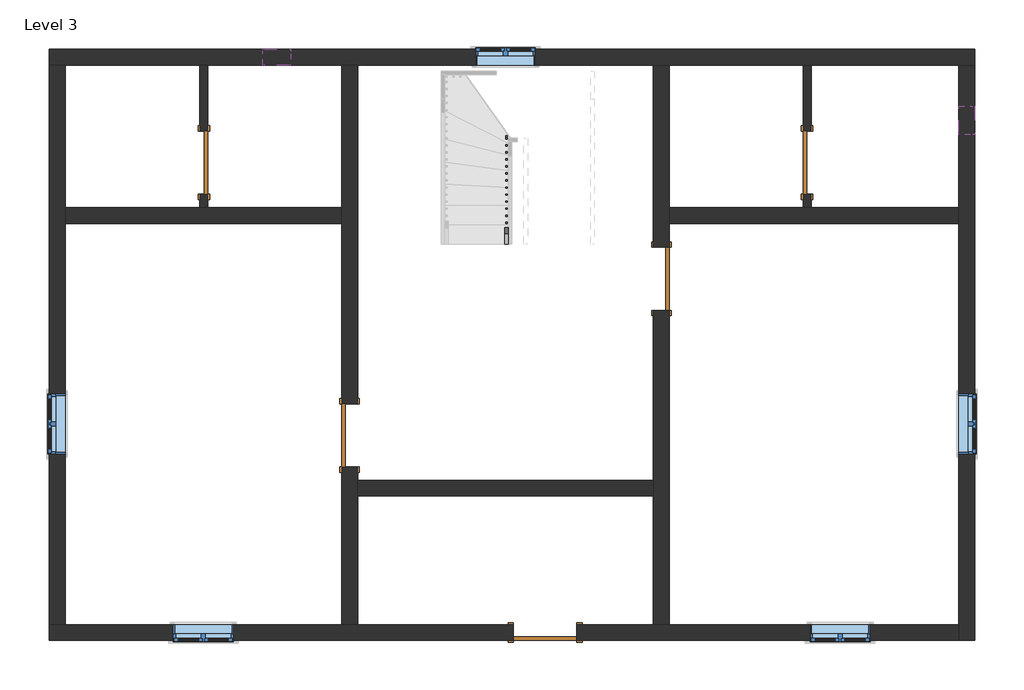
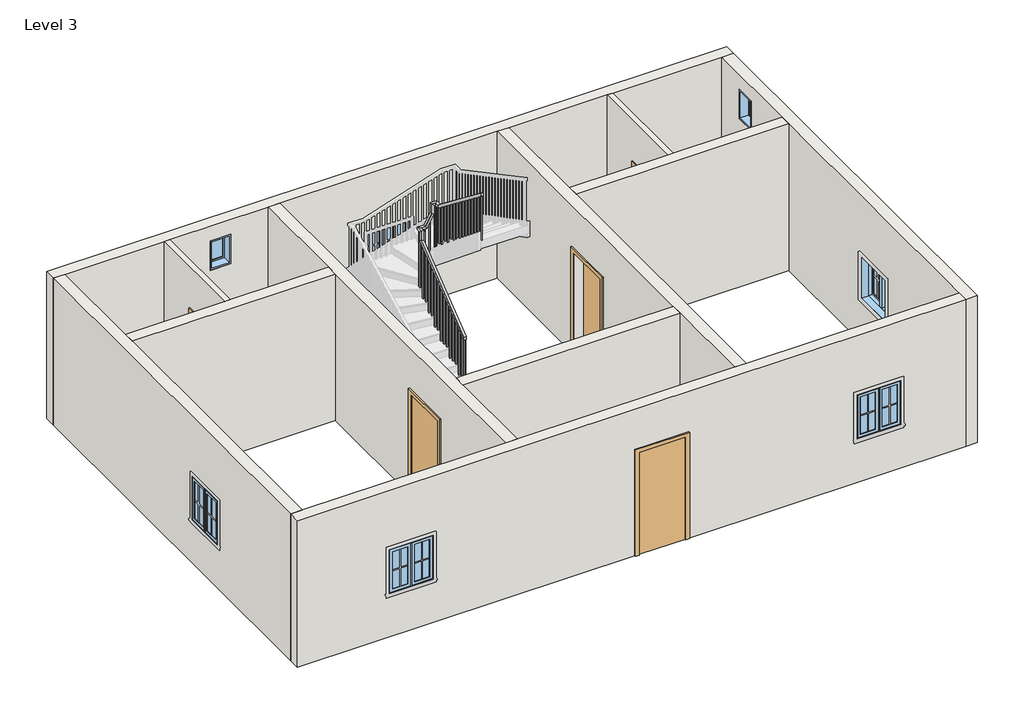
# One storey, part 1 of 2: 11 walls, 7 windows, 5 doors, 1 railing.
"""IFC4 building model written with IfcOpenShell, lengths in millimetres."""

from ifc_helpers import new_model, si_unit, frame, origin, place, context, project, spatial, polyline, outline, extrude, faceted_brep, transform, mapped, element, save
from components import door_e5f9f3c4, door_a90ba1ad, door_305aa2a5, door_0ca8825f, window_aa618e30, window_339605e1

model = new_model("IFC4")

# Units and contexts
model_context = context("Model", 3, world=origin())
ifc_project = project(units=[si_unit("LENGTHUNIT", "METRE", prefix="MILLI")], contexts=[model_context])

# Site, building, storey
site = spatial("IfcSite", under=ifc_project)
building = spatial("IfcBuilding", under=site)
storey = spatial("IfcBuildingStorey", under=building, Name="Level 3", Elevation=3200.4)

# Doors
placement = place(None, origin())
door_shape = door_e5f9f3c4(model_context)
element("IfcDoor", 1, ObjectType="Single-Flush : 36\" x 84\"", at=placement, inside=storey, context=model_context, shape_type="MappedRepresentation", body=[
    mapped(door_shape, transform((-5102.9390964, 4820.103532, 3200.4), x_axis=(0.0, -1.0, 0.0), y_axis=(1.0, 0.0, 0.0), z_axis=(0.0, 0.0, 1.0))),
])
door_2_shape = door_a90ba1ad(model_context)
element("IfcDoor", 2, ObjectType="Single-Flush : 36\" x 84\"", at=placement, inside=storey, context=model_context, shape_type="MappedRepresentation", body=[
    mapped(door_2_shape, transform((-3001.0890964, 883.103532, 3200.4), x_axis=(0.0, -1.0, 0.0), y_axis=(1.0, 0.0, 0.0), z_axis=(0.0, 0.0, 1.0))),
])
element("IfcDoor", 3, ObjectType="Single-Flush : 36\" x 84\"", at=placement, inside=storey, context=model_context, shape_type="MappedRepresentation", body=[
    mapped(door_2_shape, transform((1494.7109036, 3143.703532, 3200.4), x_axis=(0.0, 1.0, 0.0), y_axis=(-1.0, 0.0, 0.0), z_axis=(0.0, 0.0, 1.0))),
])
door_3_shape = door_305aa2a5(model_context)
element("IfcDoor", 4, ObjectType="Single-Flush : 36\" x 84\"", at=placement, inside=storey, context=model_context, shape_type="MappedRepresentation", body=[
    mapped(door_3_shape, transform((3596.5609036, 4820.103532, 3200.4), x_axis=(0.0, -1.0, 0.0), y_axis=(1.0, 0.0, 0.0), z_axis=(0.0, 0.0, 1.0))),
])
door_4_shape = door_0ca8825f(model_context)
element("IfcDoor", 5, ObjectType="Single-Flush : 36\" x 84\"", at=placement, inside=storey, context=model_context, shape_type="MappedRepresentation", body=[
    mapped(door_4_shape, transform((-181.6890964, -1961.696468, 3200.4), x_axis=(-1.0, 0.0, 0.0), y_axis=(0.0, -1.0, 0.0), z_axis=(0.0, 0.0, 1.0))),
])

# Railing
element("IfcRailing", 6, ObjectType="Handrail - Rectangular", at=placement, inside=storey, context=model_context, shape_type="SolidModel", body=[
    faceted_brep([(-765.8890964, 3647.9718401, 4284.1333333), (-765.8890964, 3647.9718401, 4219.8000346), (-715.0890964, 3647.9718401, 4219.8000346), (-715.0890964, 3647.9718401, 4284.1333333), (-765.8890964, 5099.503532, 5412.0191036), (-765.8890964, 5150.303532, 5387.1590024), (-715.0890964, 5150.303532, 5387.1590024), (-715.0890964, 5099.503532, 5412.0191036), (-765.8890964, 5099.503532, 5615.0281882), (-765.8890964, 5150.303532, 5564.2281882), (-715.0890964, 5150.303532, 5564.2281882), (-715.0890964, 5099.503532, 5615.0281882), (-765.8890964, 5226.503532, 5615.0281882), (-765.8890964, 5226.503532, 5564.2281882), (-715.0890964, 5175.703532, 5564.2281882), (-715.0890964, 5175.703532, 5615.0281882), (-638.8890964, 5226.503532, 5615.0281882), (-609.7677625, 5226.503532, 5564.2281882), (-609.7677625, 5175.703532, 5564.2281882), (-638.8890964, 5175.703532, 5615.0281882), (-511.8890964, 5226.503532, 5831.9051451), (-461.0890964, 5226.503532, 5818.1256424), (-461.0890964, 5175.703532, 5818.1256424), (-511.8890964, 5175.703532, 5831.9051451), (-511.8890964, 5226.503532, 6034.9142297), (-461.0890964, 5226.503532, 5984.1142297), (-461.0890964, 5175.703532, 5984.1142297), (-511.8890964, 5175.703532, 6034.9142297), (-384.8890964, 5226.503532, 6034.9142297), (-384.8890964, 5226.503532, 5984.1142297), (-435.6890964, 5175.703532, 5984.1142297), (-435.6890964, 5175.703532, 6034.9142297), (-384.8890964, 5099.503532, 6034.9142297), (-384.8890964, 5082.086864, 5984.1142297), (-435.6890964, 5082.086864, 5984.1142297), (-435.6890964, 5099.503532, 6034.9142297), (-384.8890964, 3647.9718401, 7162.8), (-435.6890964, 3647.9718401, 7162.8), (-435.6890964, 3647.9718401, 7098.4667013), (-384.8890964, 3647.9718401, 7098.4667013)], [[[0, 1, 2, 3]], [[1, 0, 4, 5]], [[2, 1, 5, 6]], [[3, 2, 6, 7]], [[0, 3, 7, 4]], [[5, 4, 8, 9]], [[6, 5, 9, 10]], [[7, 6, 10, 11]], [[4, 7, 11, 8]], [[9, 8, 12, 13]], [[10, 9, 13, 14]], [[11, 10, 14, 15]], [[8, 11, 15, 12]], [[13, 12, 16, 17]], [[14, 13, 17, 18]], [[15, 14, 18, 19]], [[12, 15, 19, 16]], [[17, 16, 20, 21]], [[18, 17, 21, 22]], [[19, 18, 22, 23]], [[16, 19, 23, 20]], [[21, 20, 24, 25]], [[22, 21, 25, 26]], [[23, 22, 26, 27]], [[20, 23, 27, 24]], [[25, 24, 28, 29]], [[26, 25, 29, 30]], [[27, 26, 30, 31]], [[24, 27, 31, 28]], [[29, 28, 32, 33]], [[30, 29, 33, 34]], [[31, 30, 34, 35]], [[28, 31, 35, 32]], [[36, 37, 38, 39]], [[33, 32, 36, 39]], [[34, 33, 39, 38]], [[35, 34, 38, 37]], [[32, 35, 37, 36]]]),
    extrude(outline(polyline([(3667.578532, 7083.2316852), (3686.628532, 7068.4292361), (3686.628532, 6079.0666667), (3667.578532, 6079.0666667), (3667.578532, 7083.2316852)])), frame((-419.8140964, 0.0, 0.0), z_axis=(1.0, 0.0, 0.0), x_axis=(0.0, 1.0, 0.0)), (0.0, 0.0, 1.0), 19.05),
    extrude(outline(polyline([(3769.178532, 7004.2852902), (3788.228532, 6989.4828411), (3788.228532, 6079.0666667), (3769.178532, 6079.0666667), (3769.178532, 7004.2852902)])), frame((-419.8140964, 0.0, 0.0), z_axis=(1.0, 0.0, 0.0), x_axis=(0.0, 1.0, 0.0)), (0.0, 0.0, 1.0), 19.05),
    extrude(outline(polyline([(3870.778532, 6925.3388952), (3889.828532, 6910.5364462), (3889.828532, 6079.0666667), (3870.778532, 6079.0666667), (3870.778532, 6925.3388952)])), frame((-419.8140964, 0.0, 0.0), z_axis=(1.0, 0.0, 0.0), x_axis=(0.0, 1.0, 0.0)), (0.0, 0.0, 1.0), 19.05),
    extrude(outline(polyline([(3972.378532, 6846.3925003), (3991.428532, 6831.5900512), (3991.428532, 5909.7333333), (3972.378532, 5909.7333333), (3972.378532, 6846.3925003)])), frame((-419.8140964, 0.0, 0.0), z_axis=(1.0, 0.0, 0.0), x_axis=(0.0, 1.0, 0.0)), (0.0, 0.0, 1.0), 19.05),
    extrude(outline(polyline([(4073.978532, 6767.4461053), (4093.028532, 6752.6436562), (4093.028532, 5909.7333333), (4073.978532, 5909.7333333), (4073.978532, 6767.4461053)])), frame((-419.8140964, 0.0, 0.0), z_axis=(1.0, 0.0, 0.0), x_axis=(0.0, 1.0, 0.0)), (0.0, 0.0, 1.0), 19.05),
    extrude(outline(polyline([(4175.578532, 6688.4997103), (4194.628532, 6673.6972613), (4194.628532, 5909.7333333), (4175.578532, 5909.7333333), (4175.578532, 6688.4997103)])), frame((-419.8140964, 0.0, 0.0), z_axis=(1.0, 0.0, 0.0), x_axis=(0.0, 1.0, 0.0)), (0.0, 0.0, 1.0), 19.05),
    extrude(outline(polyline([(4277.178532, 6609.5533154), (4296.228532, 6594.7508663), (4296.228532, 5740.4), (4277.178532, 5740.4), (4277.178532, 6609.5533154)])), frame((-419.8140964, 0.0, 0.0), z_axis=(1.0, 0.0, 0.0), x_axis=(0.0, 1.0, 0.0)), (0.0, 0.0, 1.0), 19.05),
    extrude(outline(polyline([(4378.778532, 6530.6069204), (4397.828532, 6515.8044713), (4397.828532, 5740.4), (4378.778532, 5740.4), (4378.778532, 6530.6069204)])), frame((-419.8140964, 0.0, 0.0), z_axis=(1.0, 0.0, 0.0), x_axis=(0.0, 1.0, 0.0)), (0.0, 0.0, 1.0), 19.05),
    extrude(outline(polyline([(4480.378532, 6451.6605254), (4499.428532, 6436.8580764), (4499.428532, 5571.0666667), (4480.378532, 5571.0666667), (4480.378532, 6451.6605254)])), frame((-419.8140964, 0.0, 0.0), z_axis=(1.0, 0.0, 0.0), x_axis=(0.0, 1.0, 0.0)), (0.0, 0.0, 1.0), 19.05),
    extrude(outline(polyline([(4581.978532, 6372.7141304), (4601.028532, 6357.9116814), (4601.028532, 5571.0666667), (4581.978532, 5571.0666667), (4581.978532, 6372.7141304)])), frame((-419.8140964, 0.0, 0.0), z_axis=(1.0, 0.0, 0.0), x_axis=(0.0, 1.0, 0.0)), (0.0, 0.0, 1.0), 19.05),
    extrude(outline(polyline([(4683.578532, 6293.7677355), (4702.628532, 6278.9652864), (4702.628532, 5571.0666667), (4683.578532, 5571.0666667), (4683.578532, 6293.7677355)])), frame((-419.8140964, 0.0, 0.0), z_axis=(1.0, 0.0, 0.0), x_axis=(0.0, 1.0, 0.0)), (0.0, 0.0, 1.0), 19.05),
    extrude(outline(polyline([(4785.178532, 6214.8213405), (4804.228532, 6200.0188914), (4804.228532, 5401.7333333), (4785.178532, 5401.7333333), (4785.178532, 6214.8213405)])), frame((-419.8140964, 0.0, 0.0), z_axis=(1.0, 0.0, 0.0), x_axis=(0.0, 1.0, 0.0)), (0.0, 0.0, 1.0), 19.05),
    extrude(outline(polyline([(4886.778532, 6135.8749455), (4905.828532, 6121.0724965), (4905.828532, 5401.7333333), (4886.778532, 5401.7333333), (4886.778532, 6135.8749455)])), frame((-419.8140964, 0.0, 0.0), z_axis=(1.0, 0.0, 0.0), x_axis=(0.0, 1.0, 0.0)), (0.0, 0.0, 1.0), 19.05),
    extrude(outline(polyline([(4988.378532, 6056.9285506), (5007.428532, 6042.1261015), (5007.428532, 5232.4), (4988.378532, 5232.4), (4988.378532, 6056.9285506)])), frame((-419.8140964, 0.0, 0.0), z_axis=(1.0, 0.0, 0.0), x_axis=(0.0, 1.0, 0.0)), (0.0, 0.0, 1.0), 19.05),
    extrude(outline(polyline([(5089.978532, 5977.9821556), (5109.028532, 5963.1797065), (5109.028532, 5232.4), (5089.978532, 5232.4), (5089.978532, 5977.9821556)])), frame((-419.8140964, 0.0, 0.0), z_axis=(1.0, 0.0, 0.0), x_axis=(0.0, 1.0, 0.0)), (0.0, 0.0, 1.0), 19.05),
    extrude(outline(polyline([(-445.2140964, 5191.578532), (-445.2140964, 5210.628532), (-426.1640964, 5210.628532), (-426.1640964, 5191.578532), (-445.2140964, 5191.578532)])), frame((0.0, 0.0, 4893.7333333), z_axis=(0.0, 0.0, 1.0), x_axis=(1.0, 0.0, 0.0)), (0.0, 0.0, 1.0), 1090.3808964),
    extrude(outline(polyline([(5704.26524, -527.7640964), (5671.7336964, -546.8140964), (4724.4, -546.8140964), (4724.4, -527.7640964), (5704.26524, -527.7640964)])), frame((0.0, 5191.578532, 0.0), z_axis=(0.0, 1.0, 0.0), x_axis=(0.0, 0.0, 1.0)), (0.0, 0.0, 1.0), 19.05),
    extrude(outline(polyline([(5530.7636744, -629.3640964), (5498.2321309, -648.4140964), (4555.0666667, -648.4140964), (4555.0666667, -629.3640964), (5530.7636744, -629.3640964)])), frame((0.0, 5191.578532, 0.0), z_axis=(0.0, 1.0, 0.0), x_axis=(0.0, 0.0, 1.0)), (0.0, 0.0, 1.0), 19.05),
    extrude(outline(polyline([(-730.9640964, 5162.4468401), (-750.0140964, 5162.4468401), (-750.0140964, 5181.4968401), (-730.9640964, 5181.4968401), (-730.9640964, 5162.4468401)])), frame((0.0, 0.0, 4385.7333333), z_axis=(0.0, 0.0, 1.0), x_axis=(1.0, 0.0, 0.0)), (0.0, 0.0, 1.0), 1178.4948549),
    extrude(outline(polyline([(5060.8468401, 5317.6483397), (5079.8968401, 5332.4507888), (5079.8968401, 4216.4), (5060.8468401, 4216.4), (5060.8468401, 5317.6483397)])), frame((-750.0140964, 0.0, 0.0), z_axis=(1.0, 0.0, 0.0), x_axis=(0.0, 1.0, 0.0)), (0.0, 0.0, 1.0), 19.05),
    extrude(outline(polyline([(4959.2468401, 5238.7019447), (4978.2968401, 5253.5043938), (4978.2968401, 4216.4), (4959.2468401, 4216.4), (4959.2468401, 5238.7019447)])), frame((-750.0140964, 0.0, 0.0), z_axis=(1.0, 0.0, 0.0), x_axis=(0.0, 1.0, 0.0)), (0.0, 0.0, 1.0), 19.05),
    extrude(outline(polyline([(4857.6468401, 5159.7555498), (4876.6968401, 5174.5579988), (4876.6968401, 4047.0666667), (4857.6468401, 4047.0666667), (4857.6468401, 5159.7555498)])), frame((-750.0140964, 0.0, 0.0), z_axis=(1.0, 0.0, 0.0), x_axis=(0.0, 1.0, 0.0)), (0.0, 0.0, 1.0), 19.05),
    extrude(outline(polyline([(4756.0468401, 5080.8091548), (4775.0968401, 5095.6116039), (4775.0968401, 4047.0666667), (4756.0468401, 4047.0666667), (4756.0468401, 5080.8091548)])), frame((-750.0140964, 0.0, 0.0), z_axis=(1.0, 0.0, 0.0), x_axis=(0.0, 1.0, 0.0)), (0.0, 0.0, 1.0), 19.05),
    extrude(outline(polyline([(4654.4468401, 5001.8627598), (4673.4968401, 5016.6652089), (4673.4968401, 3877.7333333), (4654.4468401, 3877.7333333), (4654.4468401, 5001.8627598)])), frame((-750.0140964, 0.0, 0.0), z_axis=(1.0, 0.0, 0.0), x_axis=(0.0, 1.0, 0.0)), (0.0, 0.0, 1.0), 19.05),
    extrude(outline(polyline([(4552.8468401, 4922.9163649), (4571.8968401, 4937.7188139), (4571.8968401, 3877.7333333), (4552.8468401, 3877.7333333), (4552.8468401, 4922.9163649)])), frame((-750.0140964, 0.0, 0.0), z_axis=(1.0, 0.0, 0.0), x_axis=(0.0, 1.0, 0.0)), (0.0, 0.0, 1.0), 19.05),
    extrude(outline(polyline([(4451.2468401, 4843.9699699), (4470.2968401, 4858.7724189), (4470.2968401, 3708.4), (4451.2468401, 3708.4), (4451.2468401, 4843.9699699)])), frame((-750.0140964, 0.0, 0.0), z_axis=(1.0, 0.0, 0.0), x_axis=(0.0, 1.0, 0.0)), (0.0, 0.0, 1.0), 19.05),
    extrude(outline(polyline([(4349.6468401, 4765.0235749), (4368.6968401, 4779.826024), (4368.6968401, 3708.4), (4349.6468401, 3708.4), (4349.6468401, 4765.0235749)])), frame((-750.0140964, 0.0, 0.0), z_axis=(1.0, 0.0, 0.0), x_axis=(0.0, 1.0, 0.0)), (0.0, 0.0, 1.0), 19.05),
    extrude(outline(polyline([(4248.0468401, 4686.0771799), (4267.0968401, 4700.879629), (4267.0968401, 3708.4), (4248.0468401, 3708.4), (4248.0468401, 4686.0771799)])), frame((-750.0140964, 0.0, 0.0), z_axis=(1.0, 0.0, 0.0), x_axis=(0.0, 1.0, 0.0)), (0.0, 0.0, 1.0), 19.05),
    extrude(outline(polyline([(4146.4468401, 4607.130785), (4165.4968401, 4621.933234), (4165.4968401, 3539.0666667), (4146.4468401, 3539.0666667), (4146.4468401, 4607.130785)])), frame((-750.0140964, 0.0, 0.0), z_axis=(1.0, 0.0, 0.0), x_axis=(0.0, 1.0, 0.0)), (0.0, 0.0, 1.0), 19.05),
    extrude(outline(polyline([(4044.8468401, 4528.18439), (4063.8968401, 4542.9868391), (4063.8968401, 3539.0666667), (4044.8468401, 3539.0666667), (4044.8468401, 4528.18439)])), frame((-750.0140964, 0.0, 0.0), z_axis=(1.0, 0.0, 0.0), x_axis=(0.0, 1.0, 0.0)), (0.0, 0.0, 1.0), 19.05),
    extrude(outline(polyline([(3943.2468401, 4449.237995), (3962.2968401, 4464.0404441), (3962.2968401, 3539.0666667), (3943.2468401, 3539.0666667), (3943.2468401, 4449.237995)])), frame((-750.0140964, 0.0, 0.0), z_axis=(1.0, 0.0, 0.0), x_axis=(0.0, 1.0, 0.0)), (0.0, 0.0, 1.0), 19.05),
    extrude(outline(polyline([(3841.6468401, 4370.2916001), (3860.6968401, 4385.0940491), (3860.6968401, 3369.7333333), (3841.6468401, 3369.7333333), (3841.6468401, 4370.2916001)])), frame((-750.0140964, 0.0, 0.0), z_axis=(1.0, 0.0, 0.0), x_axis=(0.0, 1.0, 0.0)), (0.0, 0.0, 1.0), 19.05),
    extrude(outline(polyline([(3740.0468401, 4291.3452051), (3759.0968401, 4306.1476541), (3759.0968401, 3369.7333333), (3740.0468401, 3369.7333333), (3740.0468401, 4291.3452051)])), frame((-750.0140964, 0.0, 0.0), z_axis=(1.0, 0.0, 0.0), x_axis=(0.0, 1.0, 0.0)), (0.0, 0.0, 1.0), 19.05),
    extrude(outline(polyline([(-419.8140964, 5191.578532), (-419.8140964, 5210.628532), (-400.7640964, 5210.628532), (-400.7640964, 5191.578532), (-419.8140964, 5191.578532)])), frame((0.0, 0.0, 5063.0666667), z_axis=(0.0, 0.0, 1.0), x_axis=(1.0, 0.0, 0.0)), (0.0, 0.0, 1.0), 921.0475631),
    extrude(outline(polyline([(-730.9640964, 5191.578532), (-750.0140964, 5191.578532), (-750.0140964, 5210.628532), (-730.9640964, 5210.628532), (-730.9640964, 5191.578532)])), frame((0.0, 0.0, 4385.7333333), z_axis=(0.0, 0.0, 1.0), x_axis=(1.0, 0.0, 0.0)), (0.0, 0.0, 1.0), 1178.4948549),
    extrude(outline(polyline([(3647.9718401, 7098.4667013), (3667.0218401, 7083.6642523), (3667.0218401, 6079.0666667), (3647.9718401, 6079.0666667), (3647.9718401, 7098.4667013)])), frame((-419.8140964, 0.0, 0.0), z_axis=(1.0, 0.0, 0.0), x_axis=(0.0, 1.0, 0.0)), (0.0, 0.0, 1.0), 19.05),
    extrude(outline(polyline([(3647.9718401, 4219.8000346), (3667.0218401, 4234.6024837), (3667.0218401, 3369.7333333), (3647.9718401, 3369.7333333), (3647.9718401, 4219.8000346)])), frame((-750.0140964, 0.0, 0.0), z_axis=(1.0, 0.0, 0.0), x_axis=(0.0, 1.0, 0.0)), (0.0, 0.0, 1.0), 19.05),
])

# Walls
element("IfcWall", 7, ObjectType="WALL4.5\"", at=placement, inside=storey, context=model_context, shape_type="SweptSolid", body=[
    extrude(outline(polyline([(4362.903532, 5334.0), (4362.903532, 3200.4), (4172.403532, 3200.4), (4172.403532, 6248.4), (6229.803532, 6248.4), (6229.803532, 3200.4), (5277.303532, 3200.4), (5277.303532, 5334.0), (4362.903532, 5334.0)])), frame((-5160.0890964, 0.0, 0.0), z_axis=(1.0, 0.0, 0.0), x_axis=(0.0, 1.0, 0.0)), (0.0, 0.0, 1.0), 114.3),
])
element("IfcWall", 8, ObjectType="WALL4.5\"", at=placement, inside=storey, context=model_context, shape_type="SweptSolid", body=[
    extrude(outline(polyline([(4362.903532, 5334.0), (4362.903532, 3200.4), (4172.403532, 3200.4), (4172.403532, 6248.4), (6229.803532, 6248.4), (6229.803532, 3200.4), (5277.303532, 3200.4), (5277.303532, 5334.0), (4362.903532, 5334.0)])), frame((3539.4109036, 0.0, 0.0), z_axis=(1.0, 0.0, 0.0), x_axis=(0.0, 1.0, 0.0)), (0.0, 0.0, 1.0), 114.3),
])
element("IfcWall", 9, ObjectType="WALL9\"", at=placement, inside=storey, context=model_context, shape_type="Brep", body=[
    faceted_brep([(-7334.9640964, 6229.803532, 3200.4), (-7106.3640964, 6229.803532, 3200.4), (-5160.0890964, 6229.803532, 3200.4), (-5045.7890964, 6229.803532, 3200.4), (-3115.3890964, 6229.803532, 3200.4), (-2886.7890964, 6229.803532, 3200.4), (1380.4109036, 6229.803532, 3200.4), (1609.0109036, 6229.803532, 3200.4), (3539.4109036, 6229.803532, 3200.4), (3653.7109036, 6229.803532, 3200.4), (5787.3109036, 6229.803532, 3200.4), (6015.9109036, 6229.803532, 3200.4), (6015.9109036, 6229.803532, 6248.4), (5787.3109036, 6229.803532, 6248.4), (3653.7109036, 6229.803532, 6248.4), (3539.4109036, 6229.803532, 6248.4), (1609.0109036, 6229.803532, 6248.4), (1380.4109036, 6229.803532, 6248.4), (-2886.7890964, 6229.803532, 6248.4), (-3115.3890964, 6229.803532, 6248.4), (-5045.7890964, 6229.803532, 6248.4), (-5160.0890964, 6229.803532, 6248.4), (-7106.3640964, 6229.803532, 6248.4), (-7334.9640964, 6229.803532, 6248.4), (-3848.8140964, 6229.803532, 5943.6), (-3848.8140964, 6229.803532, 5334.0), (-4255.2140964, 6229.803532, 5334.0), (-4255.2140964, 6229.803532, 5943.6), (-321.3890964, 6229.803532, 5029.2), (-321.3890964, 6229.803532, 4114.8), (-1184.9890964, 6229.803532, 4114.8), (-1184.9890964, 6229.803532, 5029.2), (-7334.9640964, 6458.403532, 3200.4), (-7334.9640964, 6458.403532, 6248.4), (6015.9109036, 6458.403532, 6248.4), (6015.9109036, 6458.403532, 3200.4), (-3848.8140964, 6458.403532, 5943.6), (-4255.2140964, 6458.403532, 5943.6), (-4255.2140964, 6458.403532, 5334.0), (-3848.8140964, 6458.403532, 5334.0), (-321.3890964, 6458.403532, 5029.2), (-1184.9890964, 6458.403532, 5029.2), (-1184.9890964, 6458.403532, 4114.8), (-321.3890964, 6458.403532, 4114.8)], [[[0, 1, 2, 3, 4, 5, 6, 7, 8, 9, 10, 11, 12, 13, 14, 15, 16, 17, 18, 19, 20, 21, 22, 23], [24, 25, 26, 27], [28, 29, 30, 31]], [[32, 33, 34, 35], [36, 37, 38, 39], [40, 41, 42, 43]], [[11, 10, 9, 8, 7, 6, 5, 4, 3, 2, 1, 0, 32, 35]], [[12, 11, 35, 34]], [[0, 23, 33, 32]], [[25, 24, 36, 39]], [[26, 25, 39, 38]], [[27, 26, 38, 37]], [[24, 27, 37, 36]], [[29, 28, 40, 43]], [[30, 29, 43, 42]], [[31, 30, 42, 41]], [[28, 31, 41, 40]], [[23, 22, 21, 20, 19, 18, 17, 16, 15, 14, 13, 12, 34, 33]]]),
])
element("IfcWall", 10, ObjectType="WALL9\"", at=placement, inside=storey, context=model_context, shape_type="Brep", body=[
    faceted_brep([(5787.3109036, 6229.803532, 3200.4), (5787.3109036, 4172.403532, 3200.4), (5787.3109036, 3943.803532, 3200.4), (5787.3109036, -1847.396468, 3200.4), (5787.3109036, -2075.996468, 3200.4), (5787.3109036, -2075.996468, 6248.4), (5787.3109036, -1847.396468, 6248.4), (5787.3109036, 3943.803532, 6248.4), (5787.3109036, 4172.403532, 6248.4), (5787.3109036, 6229.803532, 6248.4), (5787.3109036, 5226.503532, 5943.6), (5787.3109036, 5226.503532, 5334.0), (5787.3109036, 5632.903532, 5334.0), (5787.3109036, 5632.903532, 5943.6), (5787.3109036, 616.403532, 5029.2), (5787.3109036, 616.403532, 4114.8), (5787.3109036, 1480.003532, 4114.8), (5787.3109036, 1480.003532, 5029.2), (6015.9109036, 6229.803532, 3200.4), (6015.9109036, 6229.803532, 6248.4), (6015.9109036, -2075.996468, 6248.4), (6015.9109036, -2075.996468, 3200.4), (6015.9109036, 5226.503532, 5943.6), (6015.9109036, 5632.903532, 5943.6), (6015.9109036, 5632.903532, 5334.0), (6015.9109036, 5226.503532, 5334.0), (6015.9109036, 616.403532, 5029.2), (6015.9109036, 1480.003532, 5029.2), (6015.9109036, 1480.003532, 4114.8), (6015.9109036, 616.403532, 4114.8)], [[[0, 1, 2, 3, 4, 5, 6, 7, 8, 9], [10, 11, 12, 13], [14, 15, 16, 17]], [[18, 19, 20, 21], [22, 23, 24, 25], [26, 27, 28, 29]], [[4, 3, 2, 1, 0, 18, 21]], [[0, 9, 19, 18]], [[5, 4, 21, 20]], [[11, 10, 22, 25]], [[12, 11, 25, 24]], [[13, 12, 24, 23]], [[10, 13, 23, 22]], [[15, 14, 26, 29]], [[16, 15, 29, 28]], [[17, 16, 28, 27]], [[14, 17, 27, 26]], [[9, 8, 7, 6, 5, 20, 19]]]),
])
element("IfcWall", 11, ObjectType="WALL9\"", at=placement, inside=storey, context=model_context, shape_type="Brep", body=[
    faceted_brep([(-638.8890964, -1847.396468, 5334.0), (-638.8890964, -1847.396468, 3200.4), (-2886.7890964, -1847.396468, 3200.4), (-3115.3890964, -1847.396468, 3200.4), (-7106.3640964, -1847.396468, 3200.4), (-7334.9640964, -1847.396468, 3200.4), (-7334.9640964, -1847.396468, 6248.4), (-7106.3640964, -1847.396468, 6248.4), (-3115.3890964, -1847.396468, 6248.4), (-2886.7890964, -1847.396468, 6248.4), (1380.4109036, -1847.396468, 6248.4), (1609.0109036, -1847.396468, 6248.4), (5787.3109036, -1847.396468, 6248.4), (5787.3109036, -1847.396468, 3200.4), (1609.0109036, -1847.396468, 3200.4), (1380.4109036, -1847.396468, 3200.4), (275.5109036, -1847.396468, 3200.4), (275.5109036, -1847.396468, 5334.0), (-5542.6765964, -1847.396468, 5029.2), (-5542.6765964, -1847.396468, 4114.8), (-4679.0765964, -1847.396468, 4114.8), (-4679.0765964, -1847.396468, 5029.2), (3641.0109036, -1847.396468, 5029.2), (3641.0109036, -1847.396468, 4114.8), (4504.6109036, -1847.396468, 4114.8), (4504.6109036, -1847.396468, 5029.2), (-7334.9640964, -2075.996468, 3200.4), (-638.8890964, -2075.996468, 3200.4), (-638.8890964, -2075.996468, 5334.0), (275.5109036, -2075.996468, 5334.0), (275.5109036, -2075.996468, 3200.4), (5787.3109036, -2075.996468, 3200.4), (5787.3109036, -2075.996468, 6248.4), (-7334.9640964, -2075.996468, 6248.4), (-5542.6765964, -2075.996468, 5029.2), (-4679.0765964, -2075.996468, 5029.2), (-4679.0765964, -2075.996468, 4114.8), (-5542.6765964, -2075.996468, 4114.8), (3641.0109036, -2075.996468, 5029.2), (4504.6109036, -2075.996468, 5029.2), (4504.6109036, -2075.996468, 4114.8), (3641.0109036, -2075.996468, 4114.8)], [[[0, 1, 2, 3, 4, 5, 6, 7, 8, 9, 10, 11, 12, 13, 14, 15, 16, 17], [18, 19, 20, 21], [22, 23, 24, 25]], [[26, 27, 28, 29, 30, 31, 32, 33], [34, 35, 36, 37], [38, 39, 40, 41]], [[5, 4, 3, 2, 1, 27, 26]], [[16, 15, 14, 13, 31, 30]], [[13, 12, 32, 31]], [[6, 5, 26, 33]], [[19, 18, 34, 37]], [[20, 19, 37, 36]], [[21, 20, 36, 35]], [[18, 21, 35, 34]], [[23, 22, 38, 41]], [[24, 23, 41, 40]], [[25, 24, 40, 39]], [[22, 25, 39, 38]], [[12, 11, 10, 9, 8, 7, 6, 33, 32]], [[28, 27, 1, 0]], [[29, 28, 0, 17]], [[30, 29, 17, 16]]]),
])
element("IfcWall", 12, ObjectType="WALL9\"", at=placement, inside=storey, context=model_context, shape_type="Brep", body=[
    faceted_brep([(-7106.3640964, -1847.396468, 3200.4), (-7106.3640964, 3943.803532, 3200.4), (-7106.3640964, 4172.403532, 3200.4), (-7106.3640964, 6229.803532, 3200.4), (-7106.3640964, 6229.803532, 6248.4), (-7106.3640964, 4172.403532, 6248.4), (-7106.3640964, 3943.803532, 6248.4), (-7106.3640964, -1847.396468, 6248.4), (-7106.3640964, 1480.003532, 5029.2), (-7106.3640964, 1480.003532, 4114.8), (-7106.3640964, 616.403532, 4114.8), (-7106.3640964, 616.403532, 5029.2), (-7334.9640964, -1847.396468, 3200.4), (-7334.9640964, -1847.396468, 6248.4), (-7334.9640964, 6229.803532, 6248.4), (-7334.9640964, 6229.803532, 3200.4), (-7334.9640964, 1480.003532, 5029.2), (-7334.9640964, 616.403532, 5029.2), (-7334.9640964, 616.403532, 4114.8), (-7334.9640964, 1480.003532, 4114.8)], [[[0, 1, 2, 3, 4, 5, 6, 7], [8, 9, 10, 11]], [[12, 13, 14, 15], [16, 17, 18, 19]], [[3, 2, 1, 0, 12, 15]], [[0, 7, 13, 12]], [[4, 3, 15, 14]], [[9, 8, 16, 19]], [[10, 9, 19, 18]], [[11, 10, 18, 17]], [[8, 11, 17, 16]], [[7, 6, 5, 4, 14, 13]]]),
])
element("IfcWall", 13, ObjectType="WALL9\"", at=placement, inside=storey, context=model_context, shape_type="Brep", body=[
    faceted_brep([(-3115.3890964, 425.903532, 5334.0), (-3115.3890964, 425.903532, 3200.4), (-3115.3890964, -1847.396468, 3200.4), (-3115.3890964, -1847.396468, 6248.4), (-3115.3890964, 3943.803532, 6248.4), (-3115.3890964, 4172.403532, 6248.4), (-3115.3890964, 6229.803532, 6248.4), (-3115.3890964, 6229.803532, 3200.4), (-3115.3890964, 4172.403532, 3200.4), (-3115.3890964, 3943.803532, 3200.4), (-3115.3890964, 1340.303532, 3200.4), (-3115.3890964, 1340.303532, 5334.0), (-2886.7890964, -1847.396468, 3200.4), (-2886.7890964, 6.803532, 3200.4), (-2886.7890964, 235.403532, 3200.4), (-2886.7890964, 425.903532, 3200.4), (-2886.7890964, 425.903532, 5334.0), (-2886.7890964, 1340.303532, 5334.0), (-2886.7890964, 1340.303532, 3200.4), (-2886.7890964, 6229.803532, 3200.4), (-2886.7890964, 6229.803532, 6248.4), (-2886.7890964, 235.403532, 6248.4), (-2886.7890964, 6.803532, 6248.4), (-2886.7890964, -1847.396468, 6248.4)], [[[0, 1, 2, 3, 4, 5, 6, 7, 8, 9, 10, 11]], [[12, 13, 14, 15, 16, 17, 18, 19, 20, 21, 22, 23]], [[2, 1, 15, 14, 13, 12]], [[10, 9, 8, 7, 19, 18]], [[7, 6, 20, 19]], [[3, 2, 12, 23]], [[16, 15, 1, 0]], [[17, 16, 0, 11]], [[18, 17, 11, 10]], [[6, 5, 4, 3, 23, 22, 21, 20]]]),
])
element("IfcWall", 14, ObjectType="WALL9\"", at=placement, inside=storey, context=model_context, shape_type="SweptSolid", body=[
    extrude(outline(polyline([(1380.4109036, 6.803532), (-2886.7890964, 6.803532), (-2886.7890964, 235.403532), (1380.4109036, 235.403532), (1380.4109036, 6.803532)])), frame((0.0, 0.0, 3200.4), z_axis=(0.0, 0.0, 1.0), x_axis=(1.0, 0.0, 0.0)), (0.0, 0.0, 1.0), 3048.0),
])
element("IfcWall", 15, ObjectType="WALL9\"", at=placement, inside=storey, context=model_context, shape_type="Brep", body=[
    faceted_brep([(1609.0109036, 3600.903532, 5334.0), (1609.0109036, 3600.903532, 3200.4), (1609.0109036, 3943.803532, 3200.4), (1609.0109036, 4172.403532, 3200.4), (1609.0109036, 6229.803532, 3200.4), (1609.0109036, 6229.803532, 6248.4), (1609.0109036, 4172.403532, 6248.4), (1609.0109036, 3943.803532, 6248.4), (1609.0109036, -1847.396468, 6248.4), (1609.0109036, -1847.396468, 3200.4), (1609.0109036, 2686.503532, 3200.4), (1609.0109036, 2686.503532, 5334.0), (1380.4109036, 6229.803532, 3200.4), (1380.4109036, 3600.903532, 3200.4), (1380.4109036, 3600.903532, 5334.0), (1380.4109036, 2686.503532, 5334.0), (1380.4109036, 2686.503532, 3200.4), (1380.4109036, 235.403532, 3200.4), (1380.4109036, 6.803532, 3200.4), (1380.4109036, -1847.396468, 3200.4), (1380.4109036, -1847.396468, 6248.4), (1380.4109036, 6.803532, 6248.4), (1380.4109036, 235.403532, 6248.4), (1380.4109036, 6229.803532, 6248.4)], [[[0, 1, 2, 3, 4, 5, 6, 7, 8, 9, 10, 11]], [[12, 13, 14, 15, 16, 17, 18, 19, 20, 21, 22, 23]], [[10, 9, 19, 18, 17, 16]], [[4, 3, 2, 1, 13, 12]], [[5, 4, 12, 23]], [[9, 8, 20, 19]], [[14, 13, 1, 0]], [[15, 14, 0, 11]], [[16, 15, 11, 10]], [[8, 7, 6, 5, 23, 22, 21, 20]]]),
])
element("IfcWall", 16, ObjectType="WALL9\"", at=placement, inside=storey, context=model_context, shape_type="Brep", body=[
    faceted_brep([(1609.0109036, 3943.803532, 3200.4), (5787.3109036, 3943.803532, 3200.4), (5787.3109036, 3943.803532, 6248.4), (1609.0109036, 3943.803532, 6248.4), (1609.0109036, 4172.403532, 3200.4), (1609.0109036, 4172.403532, 6248.4), (3539.4109036, 4172.403532, 6248.4), (3653.7109036, 4172.403532, 6248.4), (5787.3109036, 4172.403532, 6248.4), (5787.3109036, 4172.403532, 3200.4), (3653.7109036, 4172.403532, 3200.4), (3539.4109036, 4172.403532, 3200.4)], [[[0, 1, 2, 3]], [[4, 5, 6, 7, 8, 9, 10, 11]], [[1, 0, 4, 11, 10, 9]], [[2, 1, 9, 8]], [[0, 3, 5, 4]], [[3, 2, 8, 7, 6, 5]]]),
])
element("IfcWall", 17, ObjectType="WALL9\"", at=placement, inside=storey, context=model_context, shape_type="Brep", body=[
    faceted_brep([(-7106.3640964, 3943.803532, 3200.4), (-3115.3890964, 3943.803532, 3200.4), (-3115.3890964, 3943.803532, 6248.4), (-7106.3640964, 3943.803532, 6248.4), (-7106.3640964, 4172.403532, 3200.4), (-7106.3640964, 4172.403532, 6248.4), (-5160.0890964, 4172.403532, 6248.4), (-5045.7890964, 4172.403532, 6248.4), (-3115.3890964, 4172.403532, 6248.4), (-3115.3890964, 4172.403532, 3200.4), (-5045.7890964, 4172.403532, 3200.4), (-5160.0890964, 4172.403532, 3200.4)], [[[0, 1, 2, 3]], [[4, 5, 6, 7, 8, 9, 10, 11]], [[1, 0, 4, 11, 10, 9]], [[0, 3, 5, 4]], [[2, 1, 9, 8]], [[3, 2, 8, 7, 6, 5]]]),
])

# Windows
window_shape = window_aa618e30(model_context)
element("IfcWindow", 18, ObjectType="Fixed : 16\" x 24\"", at=placement, inside=storey, context=model_context, shape_type="MappedRepresentation", body=[
    mapped(window_shape, transform((-4013.9140964, 6344.103532, 4419.6), x_axis=(1.0, 0.0, 0.0), y_axis=(0.0, 1.0, 0.0), z_axis=(0.0, 0.0, 1.0))),
])
element("IfcWindow", 19, ObjectType="Fixed : 16\" x 24\"", at=placement, inside=storey, context=model_context, shape_type="MappedRepresentation", body=[
    mapped(window_shape, transform((5901.6109036, 5391.603532, 4419.6), x_axis=(0.0, -1.0, 0.0), y_axis=(1.0, 0.0, 0.0), z_axis=(0.0, 0.0, 1.0))),
])
window_2_shape = window_339605e1(model_context)
element("IfcWindow", 20, ObjectType="Window-Casement-Double : 34\" x 36\"", at=placement, inside=storey, context=model_context, shape_type="MappedRepresentation", body=[
    mapped(window_2_shape, transform((-7220.6640964, 1048.203532, 3200.4), x_axis=(0.0, 1.0, 0.0), y_axis=(-1.0, 0.0, 0.0), z_axis=(0.0, 0.0, 1.0))),
])
element("IfcWindow", 21, ObjectType="Window-Casement-Double : 34\" x 36\"", at=placement, inside=storey, context=model_context, shape_type="MappedRepresentation", body=[
    mapped(window_2_shape, transform((5901.6109036, 1048.203532, 3200.4), x_axis=(0.0, -1.0, 0.0), y_axis=(1.0, 0.0, 0.0), z_axis=(0.0, 0.0, 1.0))),
])
element("IfcWindow", 22, ObjectType="Window-Casement-Double : 34\" x 36\"", at=placement, inside=storey, context=model_context, shape_type="MappedRepresentation", body=[
    mapped(window_2_shape, transform((-753.1890964, 6344.103532, 3200.4), x_axis=(1.0, 0.0, 0.0), y_axis=(0.0, 1.0, 0.0), z_axis=(0.0, 0.0, 1.0))),
])
element("IfcWindow", 23, ObjectType="Window-Casement-Double : 34\" x 36\"", at=placement, inside=storey, context=model_context, shape_type="MappedRepresentation", body=[
    mapped(window_2_shape, transform((-5110.8765964, -1961.696468, 3200.4), x_axis=(-1.0, 0.0, 0.0), y_axis=(0.0, -1.0, 0.0), z_axis=(0.0, 0.0, 1.0))),
])
element("IfcWindow", 24, ObjectType="Window-Casement-Double : 34\" x 36\"", at=placement, inside=storey, context=model_context, shape_type="MappedRepresentation", body=[
    mapped(window_2_shape, transform((4072.8109036, -1961.696468, 3200.4), x_axis=(-1.0, 0.0, 0.0), y_axis=(0.0, -1.0, 0.0), z_axis=(0.0, 0.0, 1.0))),
])

save(model, "model.ifc")

# Revit data of these elements
# Type "Single-Flush : 36\" x 84\""
#   Type Mark = "1"
#   Construction Type Id = "MDOOR"
#   Assembly Code = "C1020"
#   Analytic Construction = "Metal"
#   Thickness = 0' - 2"
#   Heat Transfer Coefficient (U) = 0.651978 BTU/(h·ft²·°F)
#   Height = 7' - 0"
#   Trim Projection Ext = 0' - 1"
#   Trim Projection Int = 0' - 1"
#   Trim Width = 0' - 3"
#   Width = 3' - 0"
#   Define Thermal Properties by = 1
#   Define Thermal Properties by = 1
#   Door Material = Door - Panel
#   Frame Material = Door - Frame
#   Visual Light Transmittance = 0
#   Solar Heat Gain Coefficient = 0
#   Function = (empty or 0)
#   Wall Closure = (empty or 0)
# Type "Handrail - Rectangular"
#   Assembly Code = "C2010400"
#   built-in parameter 1008612 = 0.0416667 (stored number, unit not read)
#   built-in parameter 1008611 = 0.0416667 (stored number, unit not read)
#   built-in parameter 1008609 = 0.333333 (stored number, unit not read)
#   built-in parameter 1008604 = 0.166667 (stored number, unit not read)
#   built-in parameter 1008603 = 0.166667 (stored number, unit not read)
#   Railing Height = 3' - 0"
#   built-in parameter 1008630 = 2
#   built-in parameter 1008610 = 2
#   built-in parameter 1008618 = Baluster - Square : 3/4"
# Type "WALL4.5\""
#   Assembly Code = "B2010"
#   Layers, outside or top first: 0' - 4 1/2" no material (function 1)
# Type "WALL9\""
#   Assembly Code = "B2010"
#   Layers, outside or top first: 0' - 9" no material (function 1)
# Type "Fixed : 16\" x 24\""
#   Type Mark = "4"
#   Construction Type Id = "GSP4R"
#   Assembly Code = "B2020100"
#   Analytic Construction = "1/8 in Pilkington single glazing"
#   Visual Light Transmittance = 0.9
#   Solar Heat Gain Coefficient = 0.78
#   Heat Transfer Coefficient (U) = 0.6496 BTU/(h·ft²·°F)
#   Height = 2' - 0"
#   Default Sill Height = 3' - 0"
#   Width = 1' - 4"
#   Window Inset = 0' - 0 3/4"
#   Define Thermal Properties by = 1
#   Define Thermal Properties by = 1
#   Glass Pane Material = Glass
#   Sash Material = Sash
#   Wall Closure = (empty or 0)
# Type "Window-Casement-Double : 34\" x 36\""
#   Type Mark = "14"
#   Fire Rating = "0.5h"
#   Assembly Code = "B2020100"
#   Analytic Construction = "Double glazing - domestic"
#   Frame Extension [instance default] = 0' - 0 1/4"
#   Window Inset [instance default] = 0' - 0"
#   Wall Thickness [instance default] = 0' - 6"
#   Interior Wall Closure [instance default] = 0' - 2 1/4"
#   Half Width = 1' - 5"
#   Visual Light Transmittance = 0.81
#   Thermal Resistance (R) = 1.8146 (h·ft²·°F)/BTU
#   Solar Heat Gain Coefficient = 0.76
#   Rough Width = 2' - 10 1/2"
#   Rough Height = 3' - 0 1/2"
#   Height = 3' - 0"
#   Heat Transfer Coefficient (U) = 0.5511 BTU/(h·ft²·°F)
#   Exterior Wall Closure [instance default] = 0' - 1 1/4"
#   Extension Jamb [instance default] = 0' - 2 1/4"
#   Default Sill Height = 3' - 0"
#   Width = 2' - 10"
#   Define Thermal Properties by = 0
#   Muntin Visibility = yes
#   Interior Trim Visibility [instance default] = yes
#   Exterior Trim Visibility [instance default] = yes
#   Extension Jamb Visibility [instance default] = yes
#   Interior Trim Material = Wood - Stained
#   Muntin Pattern = Muntin Pattern_2x2 : Muntin Pattern_2x2
#   Interior Trim = Trim-Window-Interior-Flat : Picture Frame
#   Interior Frame Material = Wood - Stained
#   Glass Panel Material = Glass
#   Exterior Trim Material = Clad - White
#   Exterior Trim = Trim-Window-Exterior-Flat : with Sill
#   Exterior Frame Material = Clad - White
#   Wall Closure = (empty or 0)
# Elements 1, 2, 3, 4, 5 (IfcDoor, "Single-Flush : 36\" x 84\"")
#   Phase Created = New Construction
#   Materials on its faces: "Door - Frame", "Door - Panel"
# Element 6 (IfcRailing, "Handrail - Rectangular")
#   Phase Created = New Construction
# Elements 7, 8 (IfcWall, "WALL4.5\"")
#   Top Offset = 0' - 0"
#   Base Offset = 0' - 0"
#   Unconnected Height = 10' - 0"
#   wall height = 10' - 0"
#   Phase Created = New Construction
#   Base Constraint = Level 3
#   Materials on its faces: "Default Wall"
# Elements 9, 10, 11, 12 (IfcWall, "WALL9\"")
#   Top Offset = 0' - 0"
#   Base Offset = 0' - 0"
#   Unconnected Height = 10' - 0"
#   wall height = 10' - 0"
#   Phase Created = New Construction
#   Base Constraint = Level 3
#   Materials on its faces: "Default Wall", "Wood Planks"
# Elements 13, 14, 15, 16, 17 (IfcWall, "WALL9\"")
#   Top Offset = 0' - 0"
#   Base Offset = 0' - 0"
#   Unconnected Height = 10' - 0"
#   wall height = 10' - 0"
#   Phase Created = New Construction
#   Base Constraint = Level 3
#   Materials on its faces: "Default Wall"
# Element 18 (IfcWindow, "Fixed : 16\" x 24\"")
#   Mark = "8"
#   Phase Created = New Construction
#   Materials on its faces: "Sash", "Glass"
# Element 19 (IfcWindow, "Fixed : 16\" x 24\"")
#   Mark = "9"
#   Phase Created = New Construction
#   Materials on its faces: "Sash", "Glass"
# Element 20 (IfcWindow, "Window-Casement-Double : 34\" x 36\"")
#   Mark = "10"
#   Window Inset = 0' - 0"
#   Interior Wall Closure = 0' - 2 1/4"
#   Frame Extension = 0' - 0 1/4"
#   Exterior Wall Closure = 0' - 1 1/4"
#   Interior Trim Visibility = yes
#   Exterior Trim Visibility = yes
#   Phase Created = New Construction
#   Materials on its faces: "Wood - Stained", "Glass", "Clad - White"
# Element 21 (IfcWindow, "Window-Casement-Double : 34\" x 36\"")
#   Mark = "11"
#   Window Inset = 0' - 0"
#   Interior Wall Closure = 0' - 2 1/4"
#   Frame Extension = 0' - 0 1/4"
#   Exterior Wall Closure = 0' - 1 1/4"
#   Interior Trim Visibility = yes
#   Exterior Trim Visibility = yes
#   Phase Created = New Construction
#   Materials on its faces: "Wood - Stained", "Glass", "Clad - White"
# Element 22 (IfcWindow, "Window-Casement-Double : 34\" x 36\"")
#   Mark = "12"
#   Window Inset = 0' - 0"
#   Interior Wall Closure = 0' - 2 1/4"
#   Frame Extension = 0' - 0 1/4"
#   Exterior Wall Closure = 0' - 1 1/4"
#   Interior Trim Visibility = yes
#   Exterior Trim Visibility = yes
#   Phase Created = New Construction
#   Materials on its faces: "Wood - Stained", "Glass", "Clad - White"
# Element 23 (IfcWindow, "Window-Casement-Double : 34\" x 36\"")
#   Mark = "13"
#   Window Inset = 0' - 0"
#   Interior Wall Closure = 0' - 2 1/4"
#   Frame Extension = 0' - 0 1/4"
#   Exterior Wall Closure = 0' - 1 1/4"
#   Interior Trim Visibility = yes
#   Exterior Trim Visibility = yes
#   Phase Created = New Construction
#   Materials on its faces: "Wood - Stained", "Glass", "Clad - White"
# Element 24 (IfcWindow, "Window-Casement-Double : 34\" x 36\"")
#   Mark = "14"
#   Window Inset = 0' - 0"
#   Interior Wall Closure = 0' - 2 1/4"
#   Frame Extension = 0' - 0 1/4"
#   Exterior Wall Closure = 0' - 1 1/4"
#   Interior Trim Visibility = yes
#   Exterior Trim Visibility = yes
#   Phase Created = New Construction
#   Materials on its faces: "Wood - Stained", "Glass", "Clad - White"
# Materials
#   "Door - Panel": class "Wood", colour RGB 210 159 95, transparency 0, Cost = 0
#   "Door - Frame": colour RGB 118 70 51, transparency 0, Cost = 0
#   "Glass": class "Glass", colour RGB 0 128 192, transparency 0.75, Description = "Soda Lime Glass", Cost = 0
#   "Sash": class "Wood", colour RGB 224 178 126, transparency 0, Cost = 0
#   "Wood - Stained": class "Wood", colour RGB 224 178 126, transparency 0, Cost = 0
#   "Clad - White": class "Wood", colour RGB 242 242 238, transparency 0, Cost = 0
#   "Default Wall": colour RGB 128 128 128, transparency 0, Cost = 0
#   "Wood Planks": class "Wood", colour RGB 193 160 115, transparency 0, Description = "Physical material.", Cost = 0
